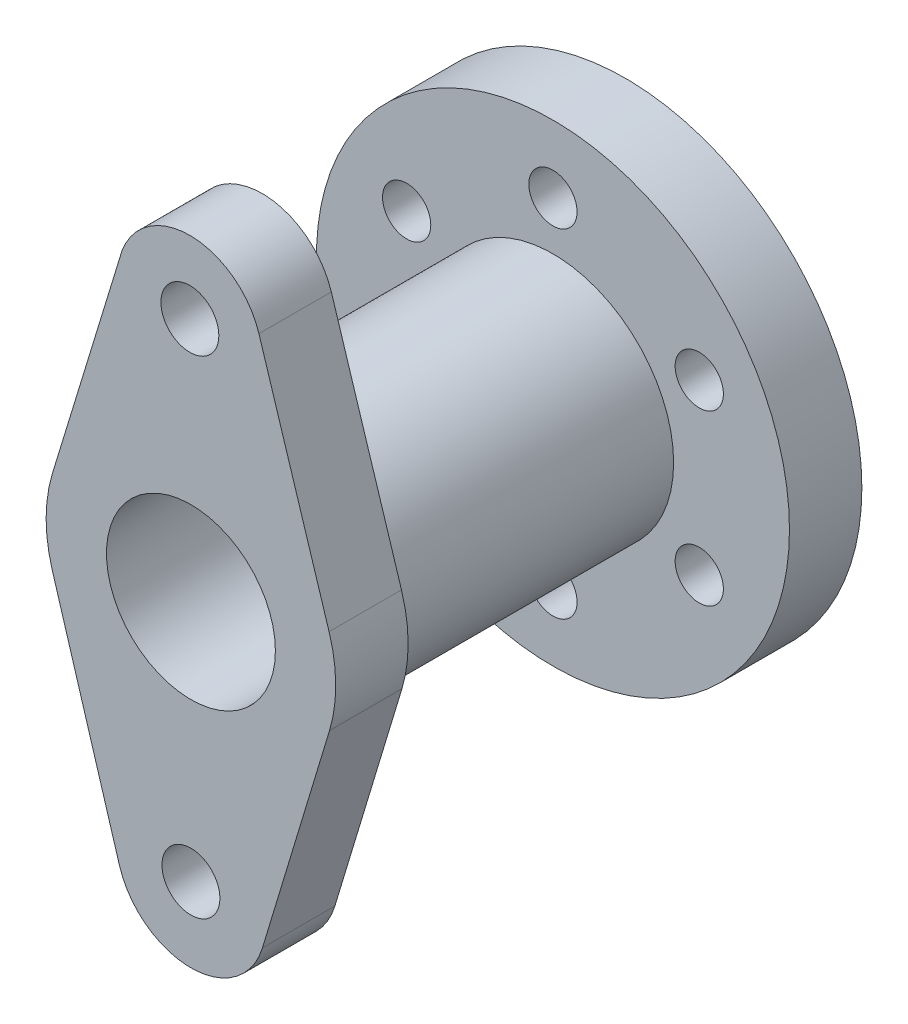
ISO-10303-21;
HEADER;
FILE_DESCRIPTION(('STEP AP214'),'2;1');
FILE_NAME('part.step','',(''),(''),'','','');
FILE_SCHEMA(('AUTOMOTIVE_DESIGN { 1 0 10303 214 1 1 1 1 }'));
ENDSEC;
DATA;
#1=APPLICATION_CONTEXT('core data for automotive mechanical design processes');
#2=APPLICATION_PROTOCOL_DEFINITION('international standard','automotive_design',2000,#1);
#3=PRODUCT_CONTEXT('',#1,'mechanical');
#4=PRODUCT('Part','Part','',(#3));
#5=PRODUCT_RELATED_PRODUCT_CATEGORY('part','',(#4));
#6=PRODUCT_DEFINITION_FORMATION('','',#4);
#7=PRODUCT_DEFINITION_CONTEXT('part definition',#1,'design');
#8=PRODUCT_DEFINITION('design','',#6,#7);
#9=PRODUCT_DEFINITION_SHAPE('','',#8);
#10=(LENGTH_UNIT() NAMED_UNIT(*) SI_UNIT(.MILLI.,.METRE.));
#11=(NAMED_UNIT(*) PLANE_ANGLE_UNIT() SI_UNIT($,.RADIAN.));
#12=(NAMED_UNIT(*) SI_UNIT($,.STERADIAN.) SOLID_ANGLE_UNIT());
#13=UNCERTAINTY_MEASURE_WITH_UNIT(LENGTH_MEASURE(1.E-05),#10,'distance_accuracy_value','');
#14=(GEOMETRIC_REPRESENTATION_CONTEXT(3) GLOBAL_UNCERTAINTY_ASSIGNED_CONTEXT((#13)) GLOBAL_UNIT_ASSIGNED_CONTEXT((#10,
#11,#12)) REPRESENTATION_CONTEXT('',''));
#15=CARTESIAN_POINT('',(0.,0.,0.));
#16=DIRECTION('',(0.,0.,1.));
#17=DIRECTION('',(1.,0.,0.));
#18=AXIS2_PLACEMENT_3D('',#15,#16,#17);
#19=CARTESIAN_POINT('',(0.,0.,15.));
#20=DIRECTION('',(0.,0.,-1.));
#21=DIRECTION('',(-1.,0.,0.));
#22=AXIS2_PLACEMENT_3D('',#19,#20,#21);
#23=CYLINDRICAL_SURFACE('',#22,49.);
#24=CARTESIAN_POINT('',(0.,0.,15.));
#25=DIRECTION('',(0.,0.,1.));
#26=DIRECTION('',(1.,0.,0.));
#27=AXIS2_PLACEMENT_3D('',#24,#25,#26);
#28=CIRCLE('',#27,49.);
#29=CARTESIAN_POINT('',(49.,0.,15.));
#30=VERTEX_POINT('',#29);
#31=EDGE_CURVE('E11',#30,#30,#28,.T.);
#32=ORIENTED_EDGE('',*,*,#31,.F.);
#33=EDGE_LOOP('',(#32));
#34=FACE_BOUND('',#33,.T.);
#35=CARTESIAN_POINT('',(0.,0.,0.));
#36=DIRECTION('',(0.,0.,1.));
#37=DIRECTION('',(1.,0.,0.));
#38=AXIS2_PLACEMENT_3D('',#35,#36,#37);
#39=CIRCLE('',#38,49.);
#40=CARTESIAN_POINT('',(49.,0.,0.));
#41=VERTEX_POINT('',#40);
#42=EDGE_CURVE('E48',#41,#41,#39,.T.);
#43=ORIENTED_EDGE('',*,*,#42,.T.);
#44=EDGE_LOOP('',(#43));
#45=FACE_BOUND('',#44,.T.);
#46=ADVANCED_FACE('F44',(#34,#45),#23,.T.);
#47=CARTESIAN_POINT('',(0.,0.,15.));
#48=DIRECTION('',(0.,0.,1.));
#49=DIRECTION('',(1.,0.,0.));
#50=AXIS2_PLACEMENT_3D('',#47,#48,#49);
#51=PLANE('',#50);
#52=CARTESIAN_POINT('',(0.,0.,15.));
#53=DIRECTION('',(0.,0.,1.));
#54=DIRECTION('',(1.,0.,0.));
#55=AXIS2_PLACEMENT_3D('',#52,#53,#54);
#56=CIRCLE('',#55,25.);
#57=CARTESIAN_POINT('',(25.,0.,15.));
#58=VERTEX_POINT('',#57);
#59=EDGE_CURVE('E175',#58,#58,#56,.T.);
#60=ORIENTED_EDGE('',*,*,#59,.F.);
#61=EDGE_LOOP('',(#60));
#62=FACE_BOUND('',#61,.T.);
#63=CARTESIAN_POINT('',(8.39071106409138E-13,34.9999999999997,15.));
#64=DIRECTION('',(0.,0.,1.));
#65=DIRECTION('',(1.,0.,0.));
#66=AXIS2_PLACEMENT_3D('',#63,#64,#65);
#67=CIRCLE('',#66,4.9999999999993);
#68=CARTESIAN_POINT('',(5.00000000000014,34.9999999999997,15.));
#69=VERTEX_POINT('',#68);
#70=EDGE_CURVE('E185',#69,#69,#67,.T.);
#71=ORIENTED_EDGE('',*,*,#70,.F.);
#72=EDGE_LOOP('',(#71));
#73=FACE_BOUND('',#72,.T.);
#74=CARTESIAN_POINT('',(-30.3108891324538,17.4999999999999,15.));
#75=DIRECTION('',(0.,0.,1.));
#76=DIRECTION('',(1.,0.,0.));
#77=AXIS2_PLACEMENT_3D('',#74,#75,#76);
#78=CIRCLE('',#77,5.0000000000001);
#79=CARTESIAN_POINT('',(-25.3108891324537,17.4999999999999,15.));
#80=VERTEX_POINT('',#79);
#81=EDGE_CURVE('E176',#80,#80,#78,.T.);
#82=ORIENTED_EDGE('',*,*,#81,.F.);
#83=EDGE_LOOP('',(#82));
#84=FACE_BOUND('',#83,.T.);
#85=CARTESIAN_POINT('',(-30.3108891324529,-17.4999999999987,15.));
#86=DIRECTION('',(0.,0.,1.));
#87=DIRECTION('',(1.,0.,0.));
#88=AXIS2_PLACEMENT_3D('',#85,#86,#87);
#89=CIRCLE('',#88,5.0000000000012);
#90=CARTESIAN_POINT('',(-25.3108891324517,-17.4999999999987,15.));
#91=VERTEX_POINT('',#90);
#92=EDGE_CURVE('E186',#91,#91,#89,.T.);
#93=ORIENTED_EDGE('',*,*,#92,.F.);
#94=EDGE_LOOP('',(#93));
#95=FACE_BOUND('',#94,.T.);
#96=CARTESIAN_POINT('',(8.39786419756654E-13,-34.9999999999978,15.));
#97=DIRECTION('',(0.,0.,1.));
#98=DIRECTION('',(1.,0.,0.));
#99=AXIS2_PLACEMENT_3D('',#96,#97,#98);
#100=CIRCLE('',#99,5.00000000000168);
#101=CARTESIAN_POINT('',(5.00000000000252,-34.9999999999978,15.));
#102=VERTEX_POINT('',#101);
#103=EDGE_CURVE('E207',#102,#102,#100,.T.);
#104=ORIENTED_EDGE('',*,*,#103,.F.);
#105=EDGE_LOOP('',(#104));
#106=FACE_BOUND('',#105,.T.);
#107=CARTESIAN_POINT('',(30.3108891324551,-17.4999999999982,15.));
#108=DIRECTION('',(0.,0.,1.));
#109=DIRECTION('',(1.,0.,0.));
#110=AXIS2_PLACEMENT_3D('',#107,#108,#109);
#111=CIRCLE('',#110,5.00000000000186);
#112=CARTESIAN_POINT('',(35.3108891324569,-17.4999999999982,15.));
#113=VERTEX_POINT('',#112);
#114=EDGE_CURVE('E197',#113,#113,#111,.T.);
#115=ORIENTED_EDGE('',*,*,#114,.F.);
#116=EDGE_LOOP('',(#115));
#117=FACE_BOUND('',#116,.T.);
#118=CARTESIAN_POINT('',(30.3108891324551,17.5000000000005,15.));
#119=DIRECTION('',(0.,0.,1.));
#120=DIRECTION('',(1.,0.,0.));
#121=AXIS2_PLACEMENT_3D('',#118,#119,#120);
#122=CIRCLE('',#121,5.00000000000062);
#123=CARTESIAN_POINT('',(35.3108891324557,17.5000000000005,15.));
#124=VERTEX_POINT('',#123);
#125=EDGE_CURVE('E191',#124,#124,#122,.T.);
#126=ORIENTED_EDGE('',*,*,#125,.F.);
#127=EDGE_LOOP('',(#126));
#128=FACE_BOUND('',#127,.T.);
#129=ORIENTED_EDGE('',*,*,#31,.T.);
#130=EDGE_LOOP('',(#129));
#131=FACE_BOUND('',#130,.T.);
#132=ADVANCED_FACE('F216',(#62,#73,#84,#95,#106,#117,#128,#131),#51,.T.);
#133=CARTESIAN_POINT('',(0.,0.,0.));
#134=DIRECTION('',(0.,0.,1.));
#135=DIRECTION('',(1.,0.,0.));
#136=AXIS2_PLACEMENT_3D('',#133,#134,#135);
#137=PLANE('',#136);
#138=CARTESIAN_POINT('',(8.39071106409138E-13,34.9999999999997,0.));
#139=DIRECTION('',(0.,0.,1.));
#140=DIRECTION('',(1.,0.,0.));
#141=AXIS2_PLACEMENT_3D('',#138,#139,#140);
#142=CIRCLE('',#141,4.9999999999993);
#143=CARTESIAN_POINT('',(5.00000000000014,34.9999999999997,0.));
#144=VERTEX_POINT('',#143);
#145=EDGE_CURVE('E177',#144,#144,#142,.T.);
#146=ORIENTED_EDGE('',*,*,#145,.T.);
#147=EDGE_LOOP('',(#146));
#148=FACE_BOUND('',#147,.T.);
#149=CARTESIAN_POINT('',(-30.3108891324538,17.4999999999999,0.));
#150=DIRECTION('',(0.,0.,1.));
#151=DIRECTION('',(1.,0.,0.));
#152=AXIS2_PLACEMENT_3D('',#149,#150,#151);
#153=CIRCLE('',#152,5.0000000000001);
#154=CARTESIAN_POINT('',(-25.3108891324537,17.4999999999999,0.));
#155=VERTEX_POINT('',#154);
#156=EDGE_CURVE('E187',#155,#155,#153,.T.);
#157=ORIENTED_EDGE('',*,*,#156,.T.);
#158=EDGE_LOOP('',(#157));
#159=FACE_BOUND('',#158,.T.);
#160=CARTESIAN_POINT('',(-30.3108891324529,-17.4999999999987,0.));
#161=DIRECTION('',(0.,0.,1.));
#162=DIRECTION('',(1.,0.,0.));
#163=AXIS2_PLACEMENT_3D('',#160,#161,#162);
#164=CIRCLE('',#163,5.0000000000012);
#165=CARTESIAN_POINT('',(-25.3108891324517,-17.4999999999987,0.));
#166=VERTEX_POINT('',#165);
#167=EDGE_CURVE('E209',#166,#166,#164,.T.);
#168=ORIENTED_EDGE('',*,*,#167,.T.);
#169=EDGE_LOOP('',(#168));
#170=FACE_BOUND('',#169,.T.);
#171=CARTESIAN_POINT('',(8.39786419756654E-13,-34.9999999999978,0.));
#172=DIRECTION('',(0.,0.,1.));
#173=DIRECTION('',(1.,0.,0.));
#174=AXIS2_PLACEMENT_3D('',#171,#172,#173);
#175=CIRCLE('',#174,5.00000000000168);
#176=CARTESIAN_POINT('',(5.00000000000252,-34.9999999999978,0.));
#177=VERTEX_POINT('',#176);
#178=EDGE_CURVE('E205',#177,#177,#175,.T.);
#179=ORIENTED_EDGE('',*,*,#178,.T.);
#180=EDGE_LOOP('',(#179));
#181=FACE_BOUND('',#180,.T.);
#182=CARTESIAN_POINT('',(30.3108891324551,-17.4999999999982,0.));
#183=DIRECTION('',(0.,0.,1.));
#184=DIRECTION('',(1.,0.,0.));
#185=AXIS2_PLACEMENT_3D('',#182,#183,#184);
#186=CIRCLE('',#185,5.00000000000186);
#187=CARTESIAN_POINT('',(35.3108891324569,-17.4999999999982,0.));
#188=VERTEX_POINT('',#187);
#189=EDGE_CURVE('E196',#188,#188,#186,.T.);
#190=ORIENTED_EDGE('',*,*,#189,.T.);
#191=EDGE_LOOP('',(#190));
#192=FACE_BOUND('',#191,.T.);
#193=CARTESIAN_POINT('',(30.3108891324551,17.5000000000005,0.));
#194=DIRECTION('',(0.,0.,1.));
#195=DIRECTION('',(1.,0.,0.));
#196=AXIS2_PLACEMENT_3D('',#193,#194,#195);
#197=CIRCLE('',#196,5.00000000000062);
#198=CARTESIAN_POINT('',(35.3108891324557,17.5000000000005,0.));
#199=VERTEX_POINT('',#198);
#200=EDGE_CURVE('E184',#199,#199,#197,.T.);
#201=ORIENTED_EDGE('',*,*,#200,.T.);
#202=EDGE_LOOP('',(#201));
#203=FACE_BOUND('',#202,.T.);
#204=ORIENTED_EDGE('',*,*,#42,.F.);
#205=EDGE_LOOP('',(#204));
#206=FACE_BOUND('',#205,.T.);
#207=ADVANCED_FACE('F217',(#148,#159,#170,#181,#192,#203,#206),#137,.F.);
#208=CARTESIAN_POINT('',(30.3108891324551,17.5000000000005,0.));
#209=DIRECTION('',(0.,0.,1.));
#210=DIRECTION('',(1.,0.,0.));
#211=AXIS2_PLACEMENT_3D('',#208,#209,#210);
#212=CYLINDRICAL_SURFACE('',#211,5.00000000000062);
#213=ORIENTED_EDGE('',*,*,#200,.F.);
#214=EDGE_LOOP('',(#213));
#215=FACE_BOUND('',#214,.T.);
#216=ORIENTED_EDGE('',*,*,#125,.T.);
#217=EDGE_LOOP('',(#216));
#218=FACE_BOUND('',#217,.T.);
#219=ADVANCED_FACE('F240',(#215,#218),#212,.F.);
#220=CARTESIAN_POINT('',(30.3108891324551,-17.4999999999982,0.));
#221=DIRECTION('',(0.,0.,1.));
#222=DIRECTION('',(1.,0.,0.));
#223=AXIS2_PLACEMENT_3D('',#220,#221,#222);
#224=CYLINDRICAL_SURFACE('',#223,5.00000000000186);
#225=ORIENTED_EDGE('',*,*,#189,.F.);
#226=EDGE_LOOP('',(#225));
#227=FACE_BOUND('',#226,.T.);
#228=ORIENTED_EDGE('',*,*,#114,.T.);
#229=EDGE_LOOP('',(#228));
#230=FACE_BOUND('',#229,.T.);
#231=ADVANCED_FACE('F243',(#227,#230),#224,.F.);
#232=CARTESIAN_POINT('',(8.39786419756654E-13,-34.9999999999978,0.));
#233=DIRECTION('',(0.,0.,1.));
#234=DIRECTION('',(1.,0.,0.));
#235=AXIS2_PLACEMENT_3D('',#232,#233,#234);
#236=CYLINDRICAL_SURFACE('',#235,5.00000000000168);
#237=ORIENTED_EDGE('',*,*,#178,.F.);
#238=EDGE_LOOP('',(#237));
#239=FACE_BOUND('',#238,.T.);
#240=ORIENTED_EDGE('',*,*,#103,.T.);
#241=EDGE_LOOP('',(#240));
#242=FACE_BOUND('',#241,.T.);
#243=ADVANCED_FACE('F252',(#239,#242),#236,.F.);
#244=CARTESIAN_POINT('',(-30.3108891324529,-17.4999999999987,0.));
#245=DIRECTION('',(0.,0.,1.));
#246=DIRECTION('',(1.,0.,0.));
#247=AXIS2_PLACEMENT_3D('',#244,#245,#246);
#248=CYLINDRICAL_SURFACE('',#247,5.0000000000012);
#249=ORIENTED_EDGE('',*,*,#167,.F.);
#250=EDGE_LOOP('',(#249));
#251=FACE_BOUND('',#250,.T.);
#252=ORIENTED_EDGE('',*,*,#92,.T.);
#253=EDGE_LOOP('',(#252));
#254=FACE_BOUND('',#253,.T.);
#255=ADVANCED_FACE('F213',(#251,#254),#248,.F.);
#256=CARTESIAN_POINT('',(-30.3108891324538,17.4999999999999,0.));
#257=DIRECTION('',(0.,0.,1.));
#258=DIRECTION('',(1.,0.,0.));
#259=AXIS2_PLACEMENT_3D('',#256,#257,#258);
#260=CYLINDRICAL_SURFACE('',#259,5.0000000000001);
#261=ORIENTED_EDGE('',*,*,#156,.F.);
#262=EDGE_LOOP('',(#261));
#263=FACE_BOUND('',#262,.T.);
#264=ORIENTED_EDGE('',*,*,#81,.T.);
#265=EDGE_LOOP('',(#264));
#266=FACE_BOUND('',#265,.T.);
#267=ADVANCED_FACE('F249',(#263,#266),#260,.F.);
#268=CARTESIAN_POINT('',(8.39071106409138E-13,34.9999999999997,0.));
#269=DIRECTION('',(0.,0.,1.));
#270=DIRECTION('',(1.,0.,0.));
#271=AXIS2_PLACEMENT_3D('',#268,#269,#270);
#272=CYLINDRICAL_SURFACE('',#271,4.9999999999993);
#273=ORIENTED_EDGE('',*,*,#145,.F.);
#274=EDGE_LOOP('',(#273));
#275=FACE_BOUND('',#274,.T.);
#276=ORIENTED_EDGE('',*,*,#70,.T.);
#277=EDGE_LOOP('',(#276));
#278=FACE_BOUND('',#277,.T.);
#279=ADVANCED_FACE('F264',(#275,#278),#272,.F.);
#280=CARTESIAN_POINT('',(0.,0.,75.));
#281=DIRECTION('',(0.,0.,-1.));
#282=DIRECTION('',(-1.,0.,0.));
#283=AXIS2_PLACEMENT_3D('',#280,#281,#282);
#284=CYLINDRICAL_SURFACE('',#283,25.);
#285=CARTESIAN_POINT('',(0.,0.,75.));
#286=DIRECTION('',(0.,0.,1.));
#287=DIRECTION('',(1.,0.,0.));
#288=AXIS2_PLACEMENT_3D('',#285,#286,#287);
#289=CIRCLE('',#288,25.);
#290=CARTESIAN_POINT('',(25.,0.,75.));
#291=VERTEX_POINT('',#290);
#292=EDGE_CURVE('E173',#291,#291,#289,.T.);
#293=ORIENTED_EDGE('',*,*,#292,.F.);
#294=EDGE_LOOP('',(#293));
#295=FACE_BOUND('',#294,.T.);
#296=ORIENTED_EDGE('',*,*,#59,.T.);
#297=EDGE_LOOP('',(#296));
#298=FACE_BOUND('',#297,.T.);
#299=ADVANCED_FACE('F262',(#295,#298),#284,.T.);
#300=CARTESIAN_POINT('',(0.,-50.1519206060856,90.));
#301=DIRECTION('',(0.,0.,-1.));
#302=DIRECTION('',(-1.,0.,0.));
#303=AXIS2_PLACEMENT_3D('',#300,#301,#302);
#304=CYLINDRICAL_SURFACE('',#303,15.475684299521);
#305=CARTESIAN_POINT('',(0.,-50.1519206060856,75.));
#306=DIRECTION('',(0.,0.,1.));
#307=DIRECTION('',(1.,0.,0.));
#308=AXIS2_PLACEMENT_3D('',#305,#306,#307);
#309=CIRCLE('',#308,15.475684299521);
#310=CARTESIAN_POINT('',(-14.8124867767712,-54.6337773671189,75.));
#311=VERTEX_POINT('',#310);
#312=CARTESIAN_POINT('',(14.8124867767712,-54.6337773671189,75.));
#313=VERTEX_POINT('',#312);
#314=EDGE_CURVE('E145',#311,#313,#309,.T.);
#315=ORIENTED_EDGE('',*,*,#314,.T.);
#316=DIRECTION('',(0.,0.,-1.));
#317=VECTOR('',#316,1.);
#318=CARTESIAN_POINT('',(14.8124867767712,-54.6337773671189,90.));
#319=LINE('',#318,#317);
#320=CARTESIAN_POINT('',(14.8124867767712,-54.6337773671189,90.));
#321=VERTEX_POINT('',#320);
#322=EDGE_CURVE('E167',#321,#313,#319,.T.);
#323=ORIENTED_EDGE('',*,*,#322,.F.);
#324=CARTESIAN_POINT('',(0.,-50.1519206060856,90.));
#325=DIRECTION('',(0.,0.,1.));
#326=DIRECTION('',(1.,0.,0.));
#327=AXIS2_PLACEMENT_3D('',#324,#325,#326);
#328=CIRCLE('',#327,15.475684299521);
#329=CARTESIAN_POINT('',(-14.8124867767712,-54.6337773671189,90.));
#330=VERTEX_POINT('',#329);
#331=EDGE_CURVE('E159',#330,#321,#328,.T.);
#332=ORIENTED_EDGE('',*,*,#331,.F.);
#333=DIRECTION('',(0.,0.,-1.));
#334=VECTOR('',#333,1.);
#335=CARTESIAN_POINT('',(-14.8124867767712,-54.6337773671189,90.));
#336=LINE('',#335,#334);
#337=EDGE_CURVE('E140',#330,#311,#336,.T.);
#338=ORIENTED_EDGE('',*,*,#337,.T.);
#339=EDGE_LOOP('',(#315,#323,#332,#338));
#340=FACE_BOUND('',#339,.T.);
#341=ADVANCED_FACE('F266',(#340),#304,.T.);
#342=CARTESIAN_POINT('',(14.8124867767712,-54.6337773671189,90.));
#343=DIRECTION('',(-0.95714583536895,0.289606370502919,0.));
#344=DIRECTION('',(-0.289606370502919,-0.957145835368951,0.));
#345=AXIS2_PLACEMENT_3D('',#342,#343,#344);
#346=PLANE('',#345);
#347=DIRECTION('',(0.289606370502919,0.95714583536895,0.));
#348=VECTOR('',#347,1.);
#349=CARTESIAN_POINT('',(14.8124867767712,-54.6337773671189,75.));
#350=LINE('',#349,#348);
#351=CARTESIAN_POINT('',(28.7143750610685,-8.68819111508758,75.));
#352=VERTEX_POINT('',#351);
#353=EDGE_CURVE('E143',#313,#352,#350,.T.);
#354=ORIENTED_EDGE('',*,*,#353,.T.);
#355=DIRECTION('',(0.,0.,-1.));
#356=VECTOR('',#355,1.);
#357=CARTESIAN_POINT('',(28.7143750610685,-8.68819111508758,90.));
#358=LINE('',#357,#356);
#359=CARTESIAN_POINT('',(28.7143750610685,-8.68819111508758,90.));
#360=VERTEX_POINT('',#359);
#361=EDGE_CURVE('E170',#360,#352,#358,.T.);
#362=ORIENTED_EDGE('',*,*,#361,.F.);
#363=DIRECTION('',(0.289606370502919,0.95714583536895,0.));
#364=VECTOR('',#363,1.);
#365=CARTESIAN_POINT('',(14.8124867767712,-54.6337773671189,90.));
#366=LINE('',#365,#364);
#367=EDGE_CURVE('E102',#321,#360,#366,.T.);
#368=ORIENTED_EDGE('',*,*,#367,.F.);
#369=ORIENTED_EDGE('',*,*,#322,.T.);
#370=EDGE_LOOP('',(#354,#362,#368,#369));
#371=FACE_BOUND('',#370,.T.);
#372=ADVANCED_FACE('F271',(#371),#346,.F.);
#373=CARTESIAN_POINT('',(0.,0.,90.));
#374=DIRECTION('',(0.,0.,-1.));
#375=DIRECTION('',(-1.,0.,0.));
#376=AXIS2_PLACEMENT_3D('',#373,#374,#375);
#377=CYLINDRICAL_SURFACE('',#376,30.);
#378=CARTESIAN_POINT('',(0.,0.,75.));
#379=DIRECTION('',(0.,0.,1.));
#380=DIRECTION('',(1.,0.,0.));
#381=AXIS2_PLACEMENT_3D('',#378,#379,#380);
#382=CIRCLE('',#381,30.);
#383=CARTESIAN_POINT('',(28.617323634226,9.00271003720396,75.));
#384=VERTEX_POINT('',#383);
#385=EDGE_CURVE('E149',#352,#384,#382,.T.);
#386=ORIENTED_EDGE('',*,*,#385,.T.);
#387=DIRECTION('',(0.,0.,-1.));
#388=VECTOR('',#387,1.);
#389=CARTESIAN_POINT('',(28.617323634226,9.00271003720396,90.));
#390=LINE('',#389,#388);
#391=CARTESIAN_POINT('',(28.617323634226,9.00271003720396,90.));
#392=VERTEX_POINT('',#391);
#393=EDGE_CURVE('E165',#392,#384,#390,.T.);
#394=ORIENTED_EDGE('',*,*,#393,.F.);
#395=CARTESIAN_POINT('',(0.,0.,90.));
#396=DIRECTION('',(0.,0.,1.));
#397=DIRECTION('',(1.,0.,0.));
#398=AXIS2_PLACEMENT_3D('',#395,#396,#397);
#399=CIRCLE('',#398,30.);
#400=EDGE_CURVE('E358',#360,#392,#399,.T.);
#401=ORIENTED_EDGE('',*,*,#400,.F.);
#402=ORIENTED_EDGE('',*,*,#361,.T.);
#403=EDGE_LOOP('',(#386,#394,#401,#402));
#404=FACE_BOUND('',#403,.T.);
#405=ADVANCED_FACE('F280',(#404),#377,.T.);
#406=CARTESIAN_POINT('',(14.0838968348735,55.2007744547682,90.));
#407=DIRECTION('',(-0.953910787807532,-0.300090334573465,0.));
#408=DIRECTION('',(0.300090334573465,-0.953910787807532,0.));
#409=AXIS2_PLACEMENT_3D('',#406,#407,#408);
#410=PLANE('',#409);
#411=DIRECTION('',(-0.300090334573465,0.953910787807532,0.));
#412=VECTOR('',#411,1.);
#413=CARTESIAN_POINT('',(14.0838968348735,55.2007744547682,75.));
#414=LINE('',#413,#412);
#415=CARTESIAN_POINT('',(14.0838968348735,55.2007744547682,75.));
#416=VERTEX_POINT('',#415);
#417=EDGE_CURVE('E148',#384,#416,#414,.T.);
#418=ORIENTED_EDGE('',*,*,#417,.T.);
#419=DIRECTION('',(0.,0.,-1.));
#420=VECTOR('',#419,1.);
#421=CARTESIAN_POINT('',(14.0838968348735,55.2007744547682,90.));
#422=LINE('',#421,#420);
#423=CARTESIAN_POINT('',(14.0838968348735,55.2007744547682,90.));
#424=VERTEX_POINT('',#423);
#425=EDGE_CURVE('E163',#424,#416,#422,.T.);
#426=ORIENTED_EDGE('',*,*,#425,.F.);
#427=DIRECTION('',(-0.300090334573465,0.953910787807532,0.));
#428=VECTOR('',#427,1.);
#429=CARTESIAN_POINT('',(14.0838968348735,55.2007744547682,90.));
#430=LINE('',#429,#428);
#431=EDGE_CURVE('E356',#392,#424,#430,.T.);
#432=ORIENTED_EDGE('',*,*,#431,.F.);
#433=ORIENTED_EDGE('',*,*,#393,.T.);
#434=EDGE_LOOP('',(#418,#426,#432,#433));
#435=FACE_BOUND('',#434,.T.);
#436=ADVANCED_FACE('F278',(#435),#410,.F.);
#437=CARTESIAN_POINT('',(-0.2204564260324,50.7007748627849,90.));
#438=DIRECTION('',(0.,0.,-1.));
#439=DIRECTION('',(-1.,0.,0.));
#440=AXIS2_PLACEMENT_3D('',#437,#438,#439);
#441=CYLINDRICAL_SURFACE('',#440,14.9954832713267);
#442=CARTESIAN_POINT('',(-0.2204564260324,50.7007748627849,75.));
#443=DIRECTION('',(0.,0.,1.));
#444=DIRECTION('',(1.,0.,0.));
#445=AXIS2_PLACEMENT_3D('',#442,#443,#444);
#446=CIRCLE('',#445,14.9954832713267);
#447=CARTESIAN_POINT('',(-14.7864897755739,54.2638060162671,75.));
#448=VERTEX_POINT('',#447);
#449=EDGE_CURVE('E151',#416,#448,#446,.T.);
#450=ORIENTED_EDGE('',*,*,#449,.T.);
#451=DIRECTION('',(0.,0.,-1.));
#452=VECTOR('',#451,1.);
#453=CARTESIAN_POINT('',(-14.7864897755739,54.2638060162671,90.));
#454=LINE('',#453,#452);
#455=CARTESIAN_POINT('',(-14.7864897755739,54.2638060162671,90.));
#456=VERTEX_POINT('',#455);
#457=EDGE_CURVE('E135',#456,#448,#454,.T.);
#458=ORIENTED_EDGE('',*,*,#457,.F.);
#459=CARTESIAN_POINT('',(-0.2204564260324,50.7007748627849,90.));
#460=DIRECTION('',(0.,0.,1.));
#461=DIRECTION('',(1.,0.,0.));
#462=AXIS2_PLACEMENT_3D('',#459,#460,#461);
#463=CIRCLE('',#462,14.9954832713267);
#464=EDGE_CURVE('E121',#424,#456,#463,.T.);
#465=ORIENTED_EDGE('',*,*,#464,.F.);
#466=ORIENTED_EDGE('',*,*,#425,.T.);
#467=EDGE_LOOP('',(#450,#458,#465,#466));
#468=FACE_BOUND('',#467,.T.);
#469=ADVANCED_FACE('F283',(#468),#441,.T.);
#470=CARTESIAN_POINT('',(-14.7864897755739,54.2638060162671,90.));
#471=DIRECTION('',(0.956339117368005,-0.292259290000823,0.));
#472=DIRECTION('',(0.292259290000823,0.956339117368005,0.));
#473=AXIS2_PLACEMENT_3D('',#470,#471,#472);
#474=PLANE('',#473);
#475=DIRECTION('',(-0.292259290000823,-0.956339117368005,0.));
#476=VECTOR('',#475,1.);
#477=CARTESIAN_POINT('',(-14.7864897755739,54.2638060162671,75.));
#478=LINE('',#477,#476);
#479=CARTESIAN_POINT('',(-28.6901735210402,8.76777870002469,75.));
#480=VERTEX_POINT('',#479);
#481=EDGE_CURVE('E131',#448,#480,#478,.T.);
#482=ORIENTED_EDGE('',*,*,#481,.T.);
#483=DIRECTION('',(0.,0.,-1.));
#484=VECTOR('',#483,1.);
#485=CARTESIAN_POINT('',(-28.6901735210402,8.76777870002469,90.));
#486=LINE('',#485,#484);
#487=CARTESIAN_POINT('',(-28.6901735210402,8.76777870002469,90.));
#488=VERTEX_POINT('',#487);
#489=EDGE_CURVE('E126',#488,#480,#486,.T.);
#490=ORIENTED_EDGE('',*,*,#489,.F.);
#491=DIRECTION('',(-0.292259290000823,-0.956339117368005,0.));
#492=VECTOR('',#491,1.);
#493=CARTESIAN_POINT('',(-14.7864897755739,54.2638060162671,90.));
#494=LINE('',#493,#492);
#495=EDGE_CURVE('E117',#456,#488,#494,.T.);
#496=ORIENTED_EDGE('',*,*,#495,.F.);
#497=ORIENTED_EDGE('',*,*,#457,.T.);
#498=EDGE_LOOP('',(#482,#490,#496,#497));
#499=FACE_BOUND('',#498,.T.);
#500=ADVANCED_FACE('F128',(#499),#474,.F.);
#501=CARTESIAN_POINT('',(0.,0.,90.));
#502=DIRECTION('',(0.,0.,-1.));
#503=DIRECTION('',(-1.,0.,0.));
#504=AXIS2_PLACEMENT_3D('',#501,#502,#503);
#505=CYLINDRICAL_SURFACE('',#504,30.);
#506=CARTESIAN_POINT('',(0.,0.,75.));
#507=DIRECTION('',(0.,0.,1.));
#508=DIRECTION('',(1.,0.,0.));
#509=AXIS2_PLACEMENT_3D('',#506,#507,#508);
#510=CIRCLE('',#509,30.);
#511=CARTESIAN_POINT('',(-28.7143750610685,-8.68819111508757,75.));
#512=VERTEX_POINT('',#511);
#513=EDGE_CURVE('E87',#480,#512,#510,.T.);
#514=ORIENTED_EDGE('',*,*,#513,.T.);
#515=DIRECTION('',(0.,0.,-1.));
#516=VECTOR('',#515,1.);
#517=CARTESIAN_POINT('',(-28.7143750610685,-8.68819111508757,90.));
#518=LINE('',#517,#516);
#519=CARTESIAN_POINT('',(-28.7143750610685,-8.68819111508757,90.));
#520=VERTEX_POINT('',#519);
#521=EDGE_CURVE('E133',#520,#512,#518,.T.);
#522=ORIENTED_EDGE('',*,*,#521,.F.);
#523=CARTESIAN_POINT('',(0.,0.,90.));
#524=DIRECTION('',(0.,0.,1.));
#525=DIRECTION('',(1.,0.,0.));
#526=AXIS2_PLACEMENT_3D('',#523,#524,#525);
#527=CIRCLE('',#526,30.);
#528=EDGE_CURVE('E125',#488,#520,#527,.T.);
#529=ORIENTED_EDGE('',*,*,#528,.F.);
#530=ORIENTED_EDGE('',*,*,#489,.T.);
#531=EDGE_LOOP('',(#514,#522,#529,#530));
#532=FACE_BOUND('',#531,.T.);
#533=ADVANCED_FACE('F137',(#532),#505,.T.);
#534=CARTESIAN_POINT('',(-14.8124867767712,-54.6337773671189,90.));
#535=DIRECTION('',(0.95714583536895,0.289606370502919,0.));
#536=DIRECTION('',(-0.289606370502919,0.95714583536895,0.));
#537=AXIS2_PLACEMENT_3D('',#534,#535,#536);
#538=PLANE('',#537);
#539=DIRECTION('',(0.289606370502919,-0.95714583536895,0.));
#540=VECTOR('',#539,1.);
#541=CARTESIAN_POINT('',(-14.8124867767712,-54.6337773671189,75.));
#542=LINE('',#541,#540);
#543=EDGE_CURVE('E98',#512,#311,#542,.T.);
#544=ORIENTED_EDGE('',*,*,#543,.T.);
#545=ORIENTED_EDGE('',*,*,#337,.F.);
#546=DIRECTION('',(0.289606370502919,-0.95714583536895,0.));
#547=VECTOR('',#546,1.);
#548=CARTESIAN_POINT('',(-14.8124867767712,-54.6337773671189,90.));
#549=LINE('',#548,#547);
#550=EDGE_CURVE('E62',#520,#330,#549,.T.);
#551=ORIENTED_EDGE('',*,*,#550,.F.);
#552=ORIENTED_EDGE('',*,*,#521,.T.);
#553=EDGE_LOOP('',(#544,#545,#551,#552));
#554=FACE_BOUND('',#553,.T.);
#555=ADVANCED_FACE('F291',(#554),#538,.F.);
#556=CARTESIAN_POINT('',(0.,-50.1519206060856,90.));
#557=DIRECTION('',(0.,0.,1.));
#558=DIRECTION('',(1.,0.,0.));
#559=AXIS2_PLACEMENT_3D('',#556,#557,#558);
#560=PLANE('',#559);
#561=CARTESIAN_POINT('',(0.,0.,90.));
#562=DIRECTION('',(0.,0.,1.));
#563=DIRECTION('',(1.,0.,0.));
#564=AXIS2_PLACEMENT_3D('',#561,#562,#563);
#565=CIRCLE('',#564,17.5);
#566=CARTESIAN_POINT('',(17.5,0.,90.));
#567=VERTEX_POINT('',#566);
#568=EDGE_CURVE('E334',#567,#567,#565,.T.);
#569=ORIENTED_EDGE('',*,*,#568,.F.);
#570=EDGE_LOOP('',(#569));
#571=FACE_BOUND('',#570,.T.);
#572=CARTESIAN_POINT('',(-0.2204564260324,50.7007748627849,90.));
#573=DIRECTION('',(0.,0.,1.));
#574=DIRECTION('',(1.,0.,0.));
#575=AXIS2_PLACEMENT_3D('',#572,#573,#574);
#576=CIRCLE('',#575,6.00000000000001);
#577=CARTESIAN_POINT('',(5.77954357396761,50.7007748627849,90.));
#578=VERTEX_POINT('',#577);
#579=EDGE_CURVE('E349',#578,#578,#576,.T.);
#580=ORIENTED_EDGE('',*,*,#579,.F.);
#581=EDGE_LOOP('',(#580));
#582=FACE_BOUND('',#581,.T.);
#583=CARTESIAN_POINT('',(0.,-50.1519206060856,90.));
#584=DIRECTION('',(0.,0.,1.));
#585=DIRECTION('',(1.,0.,0.));
#586=AXIS2_PLACEMENT_3D('',#583,#584,#585);
#587=CIRCLE('',#586,6.);
#588=CARTESIAN_POINT('',(6.00000000000001,-50.1519206060856,90.));
#589=VERTEX_POINT('',#588);
#590=EDGE_CURVE('E345',#589,#589,#587,.T.);
#591=ORIENTED_EDGE('',*,*,#590,.F.);
#592=EDGE_LOOP('',(#591));
#593=FACE_BOUND('',#592,.T.);
#594=ORIENTED_EDGE('',*,*,#331,.T.);
#595=ORIENTED_EDGE('',*,*,#367,.T.);
#596=ORIENTED_EDGE('',*,*,#400,.T.);
#597=ORIENTED_EDGE('',*,*,#431,.T.);
#598=ORIENTED_EDGE('',*,*,#464,.T.);
#599=ORIENTED_EDGE('',*,*,#495,.T.);
#600=ORIENTED_EDGE('',*,*,#528,.T.);
#601=ORIENTED_EDGE('',*,*,#550,.T.);
#602=EDGE_LOOP('',(#594,#595,#596,#597,#598,#599,#600,#601));
#603=FACE_BOUND('',#602,.T.);
#604=ADVANCED_FACE('F119',(#571,#582,#593,#603),#560,.T.);
#605=CARTESIAN_POINT('',(0.,-50.1519206060856,75.));
#606=DIRECTION('',(0.,0.,1.));
#607=DIRECTION('',(1.,0.,0.));
#608=AXIS2_PLACEMENT_3D('',#605,#606,#607);
#609=PLANE('',#608);
#610=CARTESIAN_POINT('',(-0.2204564260324,50.7007748627849,75.));
#611=DIRECTION('',(0.,0.,1.));
#612=DIRECTION('',(1.,0.,0.));
#613=AXIS2_PLACEMENT_3D('',#610,#611,#612);
#614=CIRCLE('',#613,6.00000000000001);
#615=CARTESIAN_POINT('',(5.77954357396761,50.7007748627849,75.));
#616=VERTEX_POINT('',#615);
#617=EDGE_CURVE('E147',#616,#616,#614,.T.);
#618=ORIENTED_EDGE('',*,*,#617,.T.);
#619=EDGE_LOOP('',(#618));
#620=FACE_BOUND('',#619,.T.);
#621=CARTESIAN_POINT('',(0.,-50.1519206060856,75.));
#622=DIRECTION('',(0.,0.,1.));
#623=DIRECTION('',(1.,0.,0.));
#624=AXIS2_PLACEMENT_3D('',#621,#622,#623);
#625=CIRCLE('',#624,6.);
#626=CARTESIAN_POINT('',(6.00000000000001,-50.1519206060856,75.));
#627=VERTEX_POINT('',#626);
#628=EDGE_CURVE('E348',#627,#627,#625,.T.);
#629=ORIENTED_EDGE('',*,*,#628,.T.);
#630=EDGE_LOOP('',(#629));
#631=FACE_BOUND('',#630,.T.);
#632=ORIENTED_EDGE('',*,*,#292,.T.);
#633=EDGE_LOOP('',(#632));
#634=FACE_BOUND('',#633,.T.);
#635=ORIENTED_EDGE('',*,*,#314,.F.);
#636=ORIENTED_EDGE('',*,*,#543,.F.);
#637=ORIENTED_EDGE('',*,*,#513,.F.);
#638=ORIENTED_EDGE('',*,*,#481,.F.);
#639=ORIENTED_EDGE('',*,*,#449,.F.);
#640=ORIENTED_EDGE('',*,*,#417,.F.);
#641=ORIENTED_EDGE('',*,*,#385,.F.);
#642=ORIENTED_EDGE('',*,*,#353,.F.);
#643=EDGE_LOOP('',(#635,#636,#637,#638,#639,#640,#641,#642));
#644=FACE_BOUND('',#643,.T.);
#645=ADVANCED_FACE('F298',(#620,#631,#634,#644),#609,.F.);
#646=CARTESIAN_POINT('',(0.,-50.1519206060856,75.));
#647=DIRECTION('',(0.,0.,1.));
#648=DIRECTION('',(1.,0.,0.));
#649=AXIS2_PLACEMENT_3D('',#646,#647,#648);
#650=CYLINDRICAL_SURFACE('',#649,6.);
#651=ORIENTED_EDGE('',*,*,#628,.F.);
#652=EDGE_LOOP('',(#651));
#653=FACE_BOUND('',#652,.T.);
#654=ORIENTED_EDGE('',*,*,#590,.T.);
#655=EDGE_LOOP('',(#654));
#656=FACE_BOUND('',#655,.T.);
#657=ADVANCED_FACE('F299',(#653,#656),#650,.F.);
#658=CARTESIAN_POINT('',(-0.2204564260324,50.7007748627849,75.));
#659=DIRECTION('',(0.,0.,1.));
#660=DIRECTION('',(1.,0.,0.));
#661=AXIS2_PLACEMENT_3D('',#658,#659,#660);
#662=CYLINDRICAL_SURFACE('',#661,6.00000000000001);
#663=ORIENTED_EDGE('',*,*,#617,.F.);
#664=EDGE_LOOP('',(#663));
#665=FACE_BOUND('',#664,.T.);
#666=ORIENTED_EDGE('',*,*,#579,.T.);
#667=EDGE_LOOP('',(#666));
#668=FACE_BOUND('',#667,.T.);
#669=ADVANCED_FACE('F306',(#665,#668),#662,.F.);
#670=CARTESIAN_POINT('',(0.,0.,60.));
#671=DIRECTION('',(0.,0.,1.));
#672=DIRECTION('',(1.,0.,0.));
#673=AXIS2_PLACEMENT_3D('',#670,#671,#672);
#674=CYLINDRICAL_SURFACE('',#673,17.5);
#675=CARTESIAN_POINT('',(0.,0.,60.));
#676=DIRECTION('',(0.,0.,1.));
#677=DIRECTION('',(1.,0.,0.));
#678=AXIS2_PLACEMENT_3D('',#675,#676,#677);
#679=CIRCLE('',#678,17.5);
#680=CARTESIAN_POINT('',(17.5,0.,60.));
#681=VERTEX_POINT('',#680);
#682=EDGE_CURVE('E337',#681,#681,#679,.T.);
#683=ORIENTED_EDGE('',*,*,#682,.F.);
#684=EDGE_LOOP('',(#683));
#685=FACE_BOUND('',#684,.T.);
#686=ORIENTED_EDGE('',*,*,#568,.T.);
#687=EDGE_LOOP('',(#686));
#688=FACE_BOUND('',#687,.T.);
#689=ADVANCED_FACE('F309',(#685,#688),#674,.F.);
#690=CARTESIAN_POINT('',(0.,0.,60.));
#691=DIRECTION('',(0.,0.,1.));
#692=DIRECTION('',(1.,0.,0.));
#693=AXIS2_PLACEMENT_3D('',#690,#691,#692);
#694=PLANE('',#693);
#695=CARTESIAN_POINT('',(0.,0.,60.));
#696=DIRECTION('',(0.,0.,1.));
#697=DIRECTION('',(1.,0.,0.));
#698=AXIS2_PLACEMENT_3D('',#695,#696,#697);
#699=CIRCLE('',#698,14.);
#700=CARTESIAN_POINT('',(14.,0.,60.));
#701=VERTEX_POINT('',#700);
#702=EDGE_CURVE('E335',#701,#701,#699,.T.);
#703=ORIENTED_EDGE('',*,*,#702,.F.);
#704=EDGE_LOOP('',(#703));
#705=FACE_BOUND('',#704,.T.);
#706=ORIENTED_EDGE('',*,*,#682,.T.);
#707=EDGE_LOOP('',(#706));
#708=FACE_BOUND('',#707,.T.);
#709=ADVANCED_FACE('F313',(#705,#708),#694,.T.);
#710=CARTESIAN_POINT('',(0.,0.,15.));
#711=DIRECTION('',(0.,0.,1.));
#712=DIRECTION('',(1.,0.,0.));
#713=AXIS2_PLACEMENT_3D('',#710,#711,#712);
#714=CYLINDRICAL_SURFACE('',#713,14.);
#715=CARTESIAN_POINT('',(0.,0.,15.));
#716=DIRECTION('',(0.,0.,1.));
#717=DIRECTION('',(1.,0.,0.));
#718=AXIS2_PLACEMENT_3D('',#715,#716,#717);
#719=CIRCLE('',#718,14.);
#720=CARTESIAN_POINT('',(14.,0.,15.));
#721=VERTEX_POINT('',#720);
#722=EDGE_CURVE('E332',#721,#721,#719,.T.);
#723=CARTESIAN_POINT('',(14.,0.,15.));
#724=CARTESIAN_POINT('',(14.,0.,15.46875));
#725=CARTESIAN_POINT('',(14.,0.,15.9375));
#726=CARTESIAN_POINT('',(14.,0.,16.875));
#727=CARTESIAN_POINT('',(14.,0.,17.34375));
#728=CARTESIAN_POINT('',(14.,0.,18.28125));
#729=CARTESIAN_POINT('',(14.,0.,18.75));
#730=CARTESIAN_POINT('',(14.,0.,19.6875));
#731=CARTESIAN_POINT('',(14.,0.,20.15625));
#732=CARTESIAN_POINT('',(14.,0.,21.09375));
#733=CARTESIAN_POINT('',(14.,0.,21.5625));
#734=CARTESIAN_POINT('',(14.,0.,22.5));
#735=CARTESIAN_POINT('',(14.,0.,22.96875));
#736=CARTESIAN_POINT('',(14.,0.,23.90625));
#737=CARTESIAN_POINT('',(14.,0.,24.375));
#738=CARTESIAN_POINT('',(14.,0.,25.3125));
#739=CARTESIAN_POINT('',(14.,0.,25.78125));
#740=CARTESIAN_POINT('',(14.,0.,26.71875));
#741=CARTESIAN_POINT('',(14.,0.,27.1875));
#742=CARTESIAN_POINT('',(14.,0.,28.125));
#743=CARTESIAN_POINT('',(14.,0.,28.59375));
#744=CARTESIAN_POINT('',(14.,0.,29.53125));
#745=CARTESIAN_POINT('',(14.,0.,30.));
#746=CARTESIAN_POINT('',(14.,0.,30.9375));
#747=CARTESIAN_POINT('',(14.,0.,31.40625));
#748=CARTESIAN_POINT('',(14.,0.,32.34375));
#749=CARTESIAN_POINT('',(14.,0.,32.8125));
#750=CARTESIAN_POINT('',(14.,0.,33.75));
#751=CARTESIAN_POINT('',(14.,0.,34.21875));
#752=CARTESIAN_POINT('',(14.,0.,35.15625));
#753=CARTESIAN_POINT('',(14.,0.,35.625));
#754=CARTESIAN_POINT('',(14.,0.,36.5625));
#755=CARTESIAN_POINT('',(14.,0.,37.03125));
#756=CARTESIAN_POINT('',(14.,0.,37.96875));
#757=CARTESIAN_POINT('',(14.,0.,38.4375));
#758=CARTESIAN_POINT('',(14.,0.,39.375));
#759=CARTESIAN_POINT('',(14.,0.,39.84375));
#760=CARTESIAN_POINT('',(14.,0.,40.78125));
#761=CARTESIAN_POINT('',(14.,0.,41.25));
#762=CARTESIAN_POINT('',(14.,0.,42.1875));
#763=CARTESIAN_POINT('',(14.,0.,42.65625));
#764=CARTESIAN_POINT('',(14.,0.,43.59375));
#765=CARTESIAN_POINT('',(14.,0.,44.0625));
#766=CARTESIAN_POINT('',(14.,0.,45.));
#767=CARTESIAN_POINT('',(14.,0.,45.46875));
#768=CARTESIAN_POINT('',(14.,0.,46.40625));
#769=CARTESIAN_POINT('',(14.,0.,46.875));
#770=CARTESIAN_POINT('',(14.,0.,47.8125));
#771=CARTESIAN_POINT('',(14.,0.,48.28125));
#772=CARTESIAN_POINT('',(14.,0.,49.21875));
#773=CARTESIAN_POINT('',(14.,0.,49.6875));
#774=CARTESIAN_POINT('',(14.,0.,50.625));
#775=CARTESIAN_POINT('',(14.,0.,51.09375));
#776=CARTESIAN_POINT('',(14.,0.,52.03125));
#777=CARTESIAN_POINT('',(14.,0.,52.5));
#778=CARTESIAN_POINT('',(14.,0.,53.4375));
#779=CARTESIAN_POINT('',(14.,0.,53.90625));
#780=CARTESIAN_POINT('',(14.,0.,54.84375));
#781=CARTESIAN_POINT('',(14.,0.,55.3125));
#782=CARTESIAN_POINT('',(14.,0.,56.25));
#783=CARTESIAN_POINT('',(14.,0.,56.71875));
#784=CARTESIAN_POINT('',(14.,0.,57.65625));
#785=CARTESIAN_POINT('',(14.,0.,58.125));
#786=CARTESIAN_POINT('',(14.,0.,59.0625));
#787=CARTESIAN_POINT('',(14.,0.,59.53125));
#788=CARTESIAN_POINT('',(14.,0.,60.));
#789=B_SPLINE_CURVE_WITH_KNOTS('',3,(#723,#724,#725,#726,#727,#728,#729,#730,#731,#732,#733,
#734,#735,#736,#737,#738,#739,#740,#741,#742,#743,#744,#745,#746,#747,#748,#749,#750,#751,#752,
#753,#754,#755,#756,#757,#758,#759,#760,#761,#762,#763,#764,#765,#766,#767,#768,#769,#770,#771,
#772,#773,#774,#775,#776,#777,#778,#779,#780,#781,#782,#783,#784,#785,#786,#787,#788),
.UNSPECIFIED.,.F.,.F.,(4,2,2,2,2,2,2,2,2,2,2,2,2,2,2,2,2,2,2,2,2,2,2,2,2,2,2,2,2,2,2,2,4),(0.,
1.40625,2.8125,4.21875,5.625,7.03125,8.4375,9.84375,11.25,12.65625,14.0625,15.46875,16.875,
18.28125,19.6875,21.09375,22.5,23.90625,25.3125,26.71875,28.125,29.53125,30.9375,32.34375,33.75,
35.15625,36.5625,37.96875,39.375,40.78125,42.1875,43.59375,45.),.UNSPECIFIED.);
#790=EDGE_CURVE('BSEAM319',#721,#701,#789,.T.);
#791=ORIENTED_EDGE('',*,*,#722,.F.);
#792=ORIENTED_EDGE('',*,*,#702,.T.);
#793=ORIENTED_EDGE('',*,*,#790,.T.);
#794=ORIENTED_EDGE('',*,*,#790,.F.);
#795=EDGE_LOOP('',(#791,#793,#792,#794));
#796=FACE_BOUND('',#795,.T.);
#797=ADVANCED_FACE('F319',(#796),#714,.F.);
#798=CARTESIAN_POINT('',(0.,0.,15.));
#799=DIRECTION('',(0.,0.,1.));
#800=DIRECTION('',(1.,0.,0.));
#801=AXIS2_PLACEMENT_3D('',#798,#799,#800);
#802=PLANE('',#801);
#803=ORIENTED_EDGE('',*,*,#722,.T.);
#804=EDGE_LOOP('',(#803));
#805=FACE_BOUND('',#804,.T.);
#806=ADVANCED_FACE('F325',(#805),#802,.T.);
#807=CLOSED_SHELL('',(#46,#132,#207,#219,#231,#243,#255,#267,#279,#299,#341,#372,#405,#436,#469,
#500,#533,#555,#604,#645,#657,#669,#689,#709,#797,#806));
#808=MANIFOLD_SOLID_BREP('B2',#807);
#809=ADVANCED_BREP_SHAPE_REPRESENTATION('',(#18,#808),#14);
#810=SHAPE_DEFINITION_REPRESENTATION(#9,#809);
ENDSEC;
END-ISO-10303-21;
